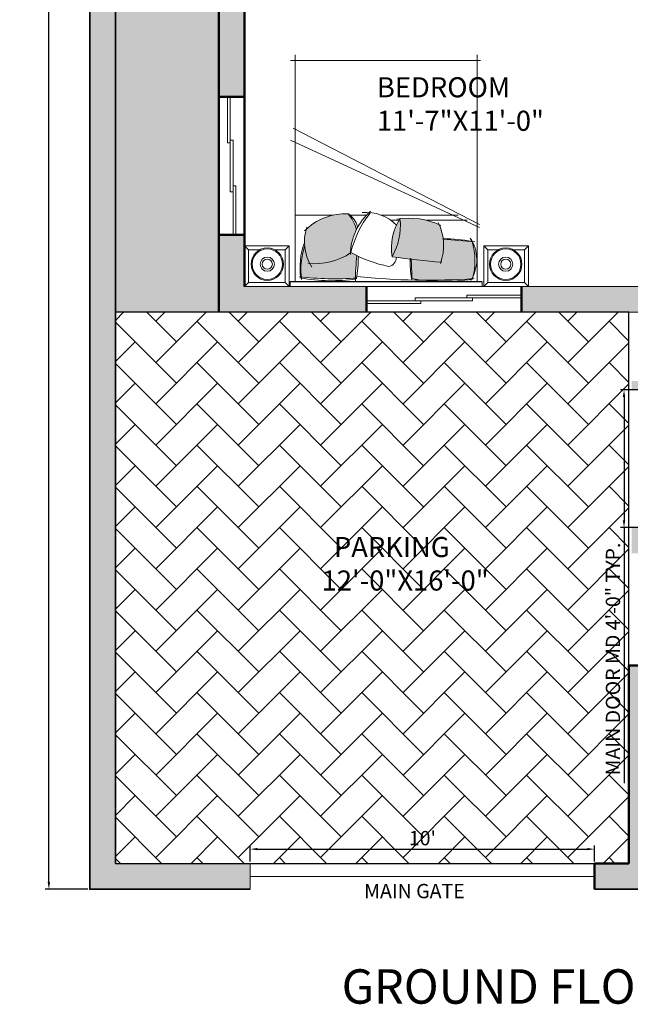
# Model space of a CAD drawing. Units: inches. Extents: x 1734 to 4011, y 1071 to 1891.
# Tile 1 of 27: x 1734 to 1947, y 1084 to 1427. Entities that reach past the tile are written whole.
import ezdxf

# ---------------------------------------------------------------- set-up
doc = ezdxf.new("R2010")
doc.units = ezdxf.units.IN
for name, color, linetype, lineweight in [('0.10', 252, 'Continuous', 9), ('0.15', 34, 'Continuous', 15), ('A-ANNO-DIMS', 2, 'Continuous', 18), ('A-ANNO-TEXT', 7, 'Continuous', 25), ('A-AREA-IDEN', 3, 'Continuous', 18), ('A-FLOR-OTLN', 7, 'Continuous', 25), ('A-FLOR-PATT', 252, 'Continuous', 13), ('A-FURN', 8, 'Continuous', 18), ('A-FURN-PATT', 252, 'Continuous', 13), ('A-GLAZ', 4, 'Continuous', 18), ('A-WALL', 7, 'Continuous', 50), ('A-WALL-PATT', 8, 'Continuous', 13), ('C-PROP', 1, 'Continuous', 35)]:
    doc.layers.add(name, color=color, linetype=linetype, lineweight=lineweight)
doc.styles.get("Standard").update_dxf_attribs({"font": 'arial.ttf'})
doc.dimstyles.new('ISO-25', dxfattribs={"dimtxt": 5, "dimasz": 2.5, "dimexe": 1.25, "dimexo": 0.625, "dimtad": 1, "dimdec": 1, "dimlunit": 3, "dimtxsty": 'Standard', "dimcen": 2.5, "dimclrt": 1, "dimadec": 0, "dimazin": 0, "dimtfac": 1, "dimtdec": 1, "dimtmove": 0, "dimatfit": 3, "dimfxl": 1, "dimarcsym": 0})

# ---------------------------------------------------------------- blocks, each defined once
blk = doc.blocks.new('*D11')
at = {"layer": 'A-ANNO-DIMS', "color": 0, "lineweight": -2, "transparency": 16777216}
for p, q in [((1814.65, 1133.69), (1814.65, 1139.29)), ((1934.65, 1133.69), (1934.65, 1139.29)), ((1817.15, 1138.04), (1932.15, 1138.04))]:
    blk.add_line(p, q, dxfattribs=at)
at = {"layer": 'A-ANNO-DIMS', "color": 0, "transparency": 16777216}
for points in [[(1817.15, 1138.46), (1817.15, 1137.63), (1814.65, 1138.04)], [(1932.15, 1138.46), (1932.15, 1137.63), (1934.65, 1138.04)]]:
    blk.add_solid(points, dxfattribs=at)
at = {"layer": 'Defpoints', "color": 0, "transparency": 16777216}
for p in [(1934.65, 1138.04), (1814.65, 1133.06), (1934.65, 1133.06)]:
    blk.add_point(p, dxfattribs=at)
at = {"layer": 'A-ANNO-DIMS', "color": 0, "transparency": 16777216, "insert": (1874.65, 1141.22), "char_height": 5, "attachment_point": 5}
blk.add_mtext("10'", dxfattribs=at)
blk = doc.blocks.new('*D15')
at = {"layer": 'A-ANNO-DIMS', "color": 0, "lineweight": -2, "transparency": 16777216}
for p, q in [((1758.02, 1844.06), (1743.18, 1844.06)), ((1744.43, 1126.56), (1744.43, 1841.56)), ((1758.02, 1124.06), (1743.18, 1124.06))]:
    blk.add_line(p, q, dxfattribs=at)
at = {"layer": 'A-ANNO-DIMS', "color": 0, "transparency": 16777216}
for points in [[(1744.01, 1841.56), (1744.84, 1841.56), (1744.43, 1844.06)], [(1744.01, 1126.56), (1744.84, 1126.56), (1744.43, 1124.06)]]:
    blk.add_solid(points, dxfattribs=at)
at = {"layer": 'Defpoints', "color": 0, "transparency": 16777216}
for p in [(1744.43, 1844.06), (1758.65, 1844.06), (1758.65, 1124.06)]:
    blk.add_point(p, dxfattribs=at)
at = {"layer": 'A-ANNO-DIMS', "color": 0, "transparency": 16777216, "insert": (1739.21, 1484.06), "char_height": 5, "attachment_point": 5, "rotation": 90}
blk.add_mtext("{\\H1.8x;60'}", dxfattribs=at)
blk = doc.blocks.new('camita')
at = {"layer": '0.10'}
for p, q in [((-0.85, -0.045), (0.85, -0.045)), ((-0.805, -0.045), (-0.805, -2.0485)), ((0.805, -0.045), (0.805, -2.0485)), ((-0.8271, -0.521), (0.8464, -1.2932)), ((-0.8271, -0.5476), (0.8236, -1.3992)), ((-0.7161, -0.585), (-0.3554, -0.585)), ((-0.1136, -0.585), (-0.0485, -0.585)), ((-0.638, -0.63), (0.0434, -0.63)), ((0.1749, -0.63), (0.3179, -0.63)), ((0.4739, -0.63), (0.805, -0.63)), ((-0.8354, -2), (0.8464, -2))]:
    blk.add_line(p, q, dxfattribs=at)
blk.add_lwpolyline([(-0.85, -0.0405), (0.85, -0.0405), (0.85, 0), (-0.85, 0)], close=True, dxfattribs=at)
for centre, radius, start, end in [((-0.4574, -0.2364), 0.3443, 147.50996, 213.83359), ((-0.1997, -0.2266), 0.5864, 163.92635, 197.14087), ((-0.3639, -5.8457), 5.7909, 83.80731, 94.12107), ((-0.5104, -1.7232), 1.6781, 80.12554, 98.66187), ((2.3534, -0.0532), 2.5803, 180.10628, 184.38541), ((-1.5443, -0.2452), 1.3333, 359.93941, 7.55329), ((1.5815, -0.2893), 1.3353, 170.38021, 178.99138), ((-1.4396, -0.0609), 1.7117, 352.92911, 0.39592), ((0.4524, -3.0675), 2.9996, 83.90257, 93.67595), ((0.4863, -1.6286), 1.5781, 80.16015, 98.05996), ((0.0294, -0.1377), 0.7262, 342.58415, 6.00484), ((0.1326, -0.1696), 0.6307, 339.92303, 8.74334), ((0.3203, -0.3944), 0.4043, 341.45245, 33.45121), ((-0.0543, -0.3633), 0.4542, 159.30257, 206.50263), ((-1.3301, -9.6748), 9.4985, 82.27078, 84.93989), ((-0.007, -0.258), 0.0828, 100.01798, 179.73597), ((-0.2931, -1.4378), 1.2903, 61.97485, 77.84351), ((0.6265, -0.7518), 0.5508, 82.96906, 124.67388), ((0.4585, -0.5454), 0.5842, 151.04555, 184.14969), ((-0.5341, -0.3393), 0.4875, 327.26442, 9.0473), ((-0.1986, -0.2742), 0.5159, 310.73945, 359.05759), ((-0.5673, -0.0868), 0.9057, 321.69527, 346.46261), ((-1.8672, -14.986), 14.6323, 84.65974, 85.75157), ((-0.4598, 1.4861), 1.9092, 260.95299, 268.65169), ((0.5707, -0.4317), 0.3145, 192.93877, 221.96363), ((0.3612, -0.133), 0.5096, 267.25889, 315.29965), ((-0.2002, 0.064), 0.6673, 244.78094, 279.06058), ((0.179, -0.272), 0.3828, 224.52836, 275.22287), ((0.4384, -0.4834), 0.1898, 193.68485, 236.70352)]:
    blk.add_arc(centre, radius, start, end, dxfattribs=at)
blk = doc.blocks.new('VELADOR')
at = {"layer": '0.15'}
for p, q in [((-0.248, 0), (-0.203, -0.045)), ((0.248, 0), (0.202, -0.045)), ((-0.203, -0.405), (-0.248, -0.45)), ((0.248, -0.45), (0.202, -0.405))]:
    blk.add_line(p, q, dxfattribs=at)
blk.add_lwpolyline([(-0.248, 0), (-0.248, -0.45), (0.248, -0.45), (0.248, 0)], close=True, dxfattribs=at)
blk.add_lwpolyline([(0.092, -0.405), (0.202, -0.405), (0.202, -0.045), (-0.203, -0.045), (-0.203, -0.405), (-0.082, -0.405)], dxfattribs=at)
for radius in [0.18, 0.169, 0.0788, 0.0563]:
    blk.add_circle((0.005, -0.247), radius, dxfattribs=at)
blk = doc.blocks.new('*D75')
at = {"layer": 'A-ANNO-DIMS', "color": 0, "lineweight": -2, "transparency": 16777216}
for p, q in [((1951.52, 1298.06), (1943.7, 1298.06)), ((1944.95, 1295.56), (1944.95, 1252.56)), ((1951.52, 1250.06), (1943.7, 1250.06)), ((1944.95, 1250.06), (1944.95, 1160.96))]:
    blk.add_line(p, q, dxfattribs=at)
at = {"layer": 'A-ANNO-DIMS', "color": 0, "transparency": 16777216}
for points in [[(1944.53, 1295.56), (1945.37, 1295.56), (1944.95, 1298.06)], [(1944.53, 1252.56), (1945.37, 1252.56), (1944.95, 1250.06)]]:
    blk.add_solid(points, dxfattribs=at)
at = {"layer": 'Defpoints', "color": 0, "transparency": 16777216}
for p in [(1952.15, 1298.06), (1944.95, 1250.06), (1952.15, 1250.06)]:
    blk.add_point(p, dxfattribs=at)
at = {"layer": 'A-ANNO-DIMS', "color": 1, "transparency": 16777216, "insert": (1941.74, 1204.26), "char_height": 5, "attachment_point": 5, "rotation": 90}
blk.add_mtext('MAIN DOOR MD 4\'-0" TYP.', dxfattribs=at)

msp = doc.modelspace()

# ---------------------------------------------------------------- hatches: boundary and pattern name
at = {"layer": 'A-FLOR-PATT'}
h = msp.add_hatch(color=256, dxfattribs=at)
h.dxf.hatch_style = 1
h.paths.add_polyline_path([(1767.65, 1758.06), (1758.65, 1758.06), (1758.65, 1124.06), (1814.65, 1124.06), (1814.65, 1133.06), (1767.65, 1133.06)])
h = msp.add_hatch(color=256, dxfattribs=at)
h.dxf.hatch_style = 1
h.paths.add_polyline_path([(1803.65, 1758.06), (1767.65, 1758.06), (1767.65, 1325.06), (1803.65, 1325.06), (1803.65, 1542.06)])
h = msp.add_hatch(dxfattribs=at)
h.set_pattern_fill('AR-HBONE', color=256, scale=0.1)
h.paths.add_polyline_path([(1946.65, 1325.06), (1767.65, 1325.06), (1767.65, 1133.06), (1946.65, 1133.06)])
h.paths.add_polyline_path([(1868.63, 1136.02), (1880.23, 1136.02), (1880.23, 1146.33), (1868.63, 1146.33)], flags=24)
h.paths.add_polyline_path([(1836.7, 1224.14), (1896.55, 1224.14), (1896.55, 1250.27), (1836.7, 1250.27)], flags=24)
at = {"layer": 'A-FURN-PATT'}
h = msp.add_hatch(color=256, dxfattribs=at)
h.dxf.hatch_style = 1
h.paths.add_polyline_path([(1851.64, 1353.83, 0.127326), (1848.78, 1359.34, 0.202559), (1834.12, 1353.96, 0.194952), (1835.4, 1342.07, 0.173835), (1849.57, 1345.73, -0.104045)])
h.paths.add_polyline_path([(1851.84, 1344.76, -0.011742), (1849.71, 1345.83, -0.175864), (1835.4, 1342.07, -0.098488), (1833.59, 1348.01, 0.094792), (1832.37, 1337.33, 0.040212), (1851.33, 1336.95, -0.029051)])
h.paths.add_polyline_path([(1880.55, 1355.57, 0.134508), (1866.82, 1357.63, 0.181694), (1864.12, 1344.4, 0.011408), (1881.07, 1342.49, 0.189536)])
h.paths.add_polyline_path([(1892.01, 1349.64, -0.004387), (1881.94, 1350.49, -0.113891), (1881.07, 1342.49, -0.006967), (1870.71, 1343.57, -0.016701), (1870.98, 1336.79, 0.015442), (1875.02, 1336.22, 0.01851), (1891.89, 1336.75, 0.020657), (1892.39, 1337.74, 0.131047)])
at = {"layer": 'A-WALL-PATT'}
h = msp.add_hatch(color=256, dxfattribs=at)
h.dxf.hatch_style = 1
h.paths.add_polyline_path([(1857.65, 1835.06), (1857.65, 1793.06), (1862.65, 1793.06), (1862.65, 1835.06), (1951.65, 1835.06), (1951.65, 1763.06), (1897.65, 1763.06), (1897.65, 1758.06), (1951.65, 1758.06), (1951.65, 1617.06), (1956.65, 1617.06), (1956.65, 1758.06), (2009.65, 1758.06), (2009.65, 1763.06), (1956.65, 1763.06), (1956.65, 1835.06), (2044.65, 1835.06), (2044.65, 1763.06), (2039.65, 1763.06), (2039.65, 1758.06), (2054.65, 1758.06), (2054.65, 1763.06), (2049.65, 1763.06), (2049.65, 1835.06), (2109.65, 1835.06), (2109.65, 1763.06), (2084.65, 1763.06), (2084.65, 1758.06), (2109.65, 1758.06), (2109.65, 1530.06), (2095.15, 1530.06), (2095.15, 1525.06), (2109.65, 1525.06), (2109.65, 1471.06), (2089.15, 1471.06), (2089.15, 1466.06), (2109.65, 1466.06), (2109.65, 1250.06), (2015.65, 1250.06), (2015.65, 1241.06), (2109.65, 1241.06), (2109.65, 1133.06), (1952.65, 1133.06), (1952.65, 1197.06), (1953.65, 1197.06), (1953.65, 1202.06), (1946.65, 1202.06), (1946.65, 1133.06), (1934.65, 1133.06), (1934.65, 1124.06), (2118.65, 1124.06), (2118.65, 1844.06), (1758.65, 1844.06), (1758.65, 1758.06), (1773.65, 1758.06), (1773.65, 1763.06), (1767.65, 1763.06), (1767.65, 1835.06)])
h.paths.add_polyline_path([(1803.65, 1649.06), (1812.65, 1649.06), (1812.65, 1758.06), (1867.65, 1758.06), (1867.65, 1763.06), (1797.65, 1763.06), (1797.65, 1758.06), (1803.65, 1758.06)], flags=17)
h.paths.add_polyline_path([(1803.65, 1572.06), (1956.65, 1572.06), (1956.65, 1581.06), (1951.65, 1581.06), (1951.65, 1577.06), (1812.65, 1577.06), (1812.65, 1601.06), (1803.65, 1601.06)], flags=17)
h.paths.add_polyline_path([(2044.65, 1530.06), (2044.65, 1525.06), (2059.15, 1525.06), (2059.15, 1530.06)], flags=17)
h.paths.add_polyline_path([(2009.65, 1466.06), (2035.15, 1466.06), (2035.15, 1471.06), (2014.65, 1471.06), (2014.65, 1530.06), (2009.65, 1530.06)], flags=17)
h.paths.add_polyline_path([(1896.65, 1537.06), (1896.65, 1533.06), (1901.65, 1533.06), (1901.65, 1542.06), (1803.65, 1542.06), (1803.65, 1507.06), (1812.65, 1507.06), (1812.65, 1537.06)], flags=17)
h.paths.add_polyline_path([(1906.65, 1466.06), (1906.65, 1471.06), (1901.65, 1471.06), (1901.65, 1503.06), (1896.65, 1503.06), (1896.65, 1471.06), (1812.65, 1471.06), (1812.65, 1483.06), (1803.65, 1483.06), (1803.65, 1400.06), (1812.65, 1400.06), (1812.65, 1466.06)], flags=17)
h.paths.add_polyline_path([(1951.65, 1334.06), (1909.15, 1334.06), (1909.15, 1325.06), (1956.65, 1325.06), (1956.65, 1466.06), (1961.65, 1466.06), (1961.65, 1471.06), (1942.65, 1471.06), (1942.65, 1466.06), (1951.65, 1466.06)], flags=17)
h.paths.add_polyline_path([(1812.65, 1334.06), (1812.65, 1352.06), (1803.65, 1352.06), (1803.65, 1325.06), (1855.15, 1325.06), (1855.15, 1334.06)], flags=17)
h.paths.add_polyline_path([(1956.65, 1298.06), (1956.65, 1301.06), (1947.65, 1301.06), (1947.65, 1298.06)], flags=17)
h.paths.add_polyline_path([(1967.65, 1241.06), (1967.65, 1250.06), (1947.65, 1250.06), (1947.65, 1241.06)], flags=17)

# ---------------------------------------------------------------- linework, layer by layer
at = {"layer": 'A-FLOR-OTLN'}
msp.add_lwpolyline([(1946.65, 1325.06), (1767.65, 1325.06), (1767.65, 1133.06), (1946.65, 1133.06)], close=True, dxfattribs=at)
at = {"layer": 'A-FURN'}
for p, q in [((1812.65, 1334.06), (1951.65, 1334.06)), ((1767.65, 1325.06), (1956.65, 1325.06)), ((1814.65, 1133.06), (1767.65, 1133.06)), ((1814.65, 1133.06), (1814.65, 1124.06)), ((1814.65, 1128.56), (1934.65, 1128.56))]:
    msp.add_line(p, q, dxfattribs=at)
at = {"layer": 'A-GLAZ'}
for p, q in [((1806.65, 1400.06), (1806.65, 1384.06)), ((1807.65, 1400.06), (1807.65, 1367.06)), ((1806.65, 1384.06), (1807.65, 1384.06)), ((1807.65, 1385.06), (1808.65, 1385.06)), ((1808.65, 1385.06), (1808.65, 1352.06)), ((1808.65, 1369.06), (1809.65, 1369.06)), ((1809.65, 1369.06), (1809.65, 1352.06)), ((1807.65, 1367.06), (1808.65, 1367.06)), ((1890.15, 1331.06), (1890.15, 1330.06)), ((1890.15, 1331.06), (1909.15, 1331.06)), ((1855.15, 1329.06), (1892.15, 1329.06)), ((1855.15, 1328.06), (1874.15, 1328.06)), ((1872.15, 1330.06), (1909.15, 1330.06)), ((1872.15, 1330.06), (1872.15, 1329.06)), ((1874.15, 1329.06), (1874.15, 1328.06)), ((1892.15, 1330.06), (1892.15, 1329.06))]:
    msp.add_line(p, q, dxfattribs=at)
at = {"layer": 'A-WALL'}
for p, q in [((1803.65, 1325.06), (1803.65, 1542.06)), ((1812.65, 1334.06), (1812.65, 1466.06)), ((1803.65, 1400.06), (1812.65, 1400.06)), ((1803.65, 1352.06), (1812.65, 1352.06)), ((1855.15, 1334.06), (1855.15, 1325.06)), ((1909.15, 1334.06), (1909.15, 1325.06)), ((1946.65, 1202.06), (1946.65, 1133.06)), ((1953.65, 1202.06), (1946.65, 1202.06)), ((1946.65, 1133.06), (1934.65, 1133.06)), ((1934.65, 1133.06), (1934.65, 1124.06))]:
    msp.add_line(p, q, dxfattribs=at)
at = {"layer": 'C-PROP'}
msp.add_line((1767.65, 1133.06), (1767.65, 1758.06), dxfattribs=at)
msp.add_lwpolyline([(1814.65, 1124.06), (1758.65, 1124.06), (1758.65, 1844.06), (2118.65, 1844.06), (2118.65, 1124.06), (1934.65, 1124.06)], dxfattribs=at)

# ---------------------------------------------------------------- block references
at = {"layer": 'A-FURN', "rotation": 180}
for name, p, xscale, yscale, zscale in [('camita', (1862.04, 1334.06), 39.375, 39.375, 39.375), ('VELADOR', (1820.42, 1334.06), -31.41542173157097, 31.41542173157097, 31.41542173157097), ('VELADOR', (1903.87, 1334.06), 31.41542173157097, 31.41542173157097, 31.41542173157097)]:
    msp.add_blockref(name, p, dxfattribs=dict(at, xscale=xscale, yscale=yscale, zscale=zscale))

# ---------------------------------------------------------------- texts
at = {"layer": 'A-ANNO-TEXT', "attachment_point": 1}
for s, width, insert, char_height in [('MAIN GATE', 86.9528, (1854.33, 1125.93), 5), ('GROUND FLOOR PLAN', 228.5661, (1846.5, 1096.19), 12)]:
    msp.add_mtext_dynamic_manual_height_columns(s, width=width, gutter_width=12.5, heights=[0], dxfattribs=dict(at, insert=insert, char_height=char_height))
at = {"layer": 'A-AREA-IDEN', "char_height": 7, "attachment_point": 1}
for s, insert in [('BEDROOM\\P11\'-7"X11\'-0"', (1858.78, 1406.93)), ('  PARKING\\P12\'-0"X16\'-0"', (1839.52, 1246.78))]:
    msp.add_mtext_dynamic_manual_height_columns(s, width=86.9528, gutter_width=12.5, heights=[0], dxfattribs=dict(at, insert=insert))

# ---------------------------------------------------------------- dimensions: what is measured, and where the dimension line sits
at = {"layer": 'A-ANNO-DIMS'}
for base, p1, p2, angle, text, override, picture, middle in [((1744.43, 1844.06), (1758.65, 1124.06), (1758.65, 1844.06), 90, '{\\H1.8x;<>}', {"dimclrd": 0, "dimclre": 0, "dimclrt": 0}, '*D15', (1739.21, 1484.06)), ((1944.95, 1250.06), (1952.15, 1298.06), (1952.15, 1250.06), 270, 'MAIN DOOR MD <> TYP.', {"dimdec": 1, "dimrnd": 0, "dimzin": 1, "dimlunit": 4, "dimfrac": 2}, '*D75', (1941.74, 1204.26))]:
    dim = msp.add_linear_dim(base=base, p1=p1, p2=p2, angle=angle, text=text, dimstyle='ISO-25', override=override, dxfattribs=at)
    dim.commit()
    dim.dimension.update_dxf_attribs({"geometry": picture, "text_midpoint": middle})
dim = msp.add_linear_dim(base=(1934.65, 1138.04), p1=(1814.65, 1133.06), p2=(1934.65, 1133.06), dimstyle='ISO-25', override={"dimclrd": 0, "dimclre": 0, "dimclrt": 0}, dxfattribs=at)
dim.commit()
dim.dimension.update_dxf_attribs({"geometry": '*D11', "text_midpoint": (1874.65, 1141.22)})

doc.saveas('drawing.dxf')
